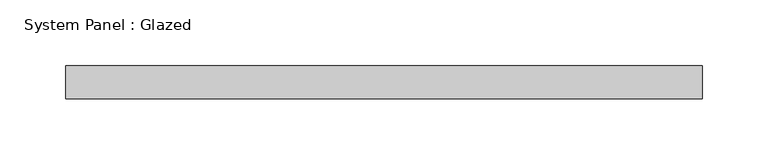
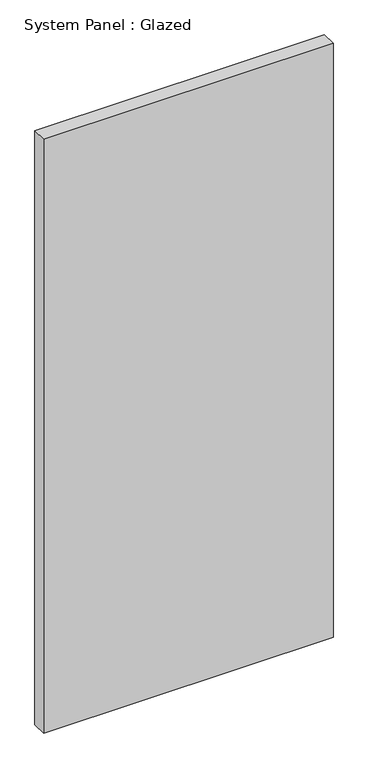
"""IFC4 building model written with IfcOpenShell, lengths in millimetres: plate geometry, System Panel : Glazed."""

from ifc_helpers import new_model, si_unit, origin, origin_with_axes, place, context, project, spatial, polyline, outline, extrude, source, transform, mapped, element, save


def system_panel_glazed_79c163db(model_context):
    return source(origin(), model_context, "Body", "SweptSolid", [
        extrude(outline(polyline([(242.1, 24.5), (-242.1, 24.5), (-242.1, 49.5), (242.1, 49.5), (242.1, 24.5)])), origin_with_axes(), (0.0, 0.0, 1.0), 1050.0),
    ])


if __name__ == "__main__":
    model = new_model("IFC4")
    model_context = context("Model", 3, world=origin())
    ifc_project = project(units=[si_unit("LENGTHUNIT", "METRE", prefix="MILLI")], contexts=[model_context])
    site = spatial("IfcSite", under=ifc_project)
    building = spatial("IfcBuilding", under=site)
    placement = place(None, origin())
    system_panel_glazed_shape = system_panel_glazed_79c163db(model_context)
    element("IfcPlate", 1, ObjectType="System Panel : Glazed", at=placement, inside=building, context=model_context, shape_type="MappedRepresentation", body=[
        mapped(system_panel_glazed_shape, transform((0.0, 0.0, 0.0), x_axis=(1.0, 0.0, 0.0), y_axis=(0.0, 1.0, 0.0), z_axis=(0.0, 0.0, 1.0))),
    ])
    save(model, "model.ifc")

# Revit data of these elements
# Type "System Panel : Glazed"
#   Keynote = "H11"
#   Construction Type Id = "GSP4R"
#   Analytic Construction = "1/8 in Pilkington single glazing"
#   Visual Light Transmittance = 0.9
#   Solar Heat Gain Coefficient = 0.86
#   Heat Transfer Coefficient (U) = 6.7069 W/(m²·K)
#   Define Thermal Properties by = 1
# Element 1 (IfcPlate, "System Panel : Glazed")
#   Materials on its faces: "Glass"
# Materials
#   "Glass": class "Glass", colour RGB 0 128 192, transparency 0.9, Description = "Soda Lime Glass", Cost = 0
